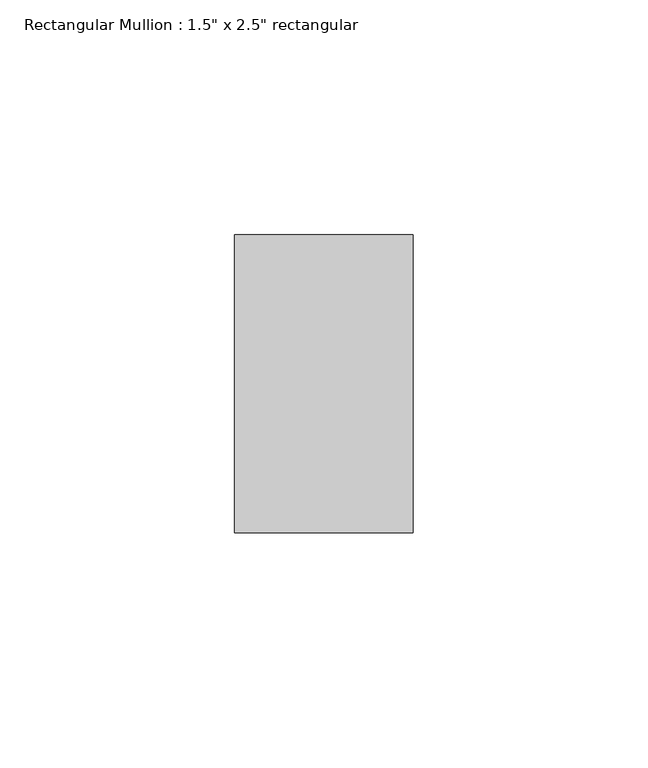
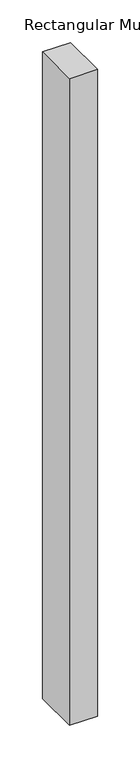
"""IFC4 building model written with IfcOpenShell, lengths in millimetres: member geometry."""

from ifc_helpers import new_model, si_unit, frame, origin, place, context, project, spatial, polyline, outline, extrude, source, transform, mapped, element, save


def member_c65a811d(model_context):
    return source(origin(), model_context, "Body", "SweptSolid", [
        extrude(outline(polyline([(0.0, 31.75), (0.0, -31.75), (-38.1, -31.75), (-38.1, 31.75), (0.0, 31.75)])), frame((0.0, 0.0, -927.1000003), z_axis=(0.0, 0.0, 1.0), x_axis=(1.0, 0.0, 0.0)), (0.0, 0.0, 1.0), 927.1000003),
    ])


if __name__ == "__main__":
    model = new_model("IFC4")
    model_context = context("Model", 3, world=origin())
    ifc_project = project(units=[si_unit("LENGTHUNIT", "METRE", prefix="MILLI")], contexts=[model_context])
    site = spatial("IfcSite", under=ifc_project)
    building = spatial("IfcBuilding", under=site)
    placement = place(None, origin())
    member_shape = member_c65a811d(model_context)
    element("IfcMember", 1, ObjectType="Rectangular Mullion : 1.5\" x 2.5\" rectangular", at=placement, inside=building, context=model_context, shape_type="MappedRepresentation", body=[
        mapped(member_shape, transform((0.0, 0.0, 0.0), x_axis=(1.0, 0.0, 0.0), y_axis=(0.0, 1.0, 0.0), z_axis=(0.0, 0.0, 1.0))),
    ])
    save(model, "model.ifc")

# Revit data of these elements
# Type "Rectangular Mullion : 1.5\" x 2.5\" rectangular"
#   built-in parameter 1007304 = 0.208333 (stored number, unit not read)
#   built-in parameter 1007301 = 0.0625 (stored number, unit not read)
#   built-in parameter 1007300 = 0.0625 (stored number, unit not read)
# Element 1 (IfcMember, "Rectangular Mullion : 1.5\" x 2.5\" rectangular")
#   Materials on its faces: "Aluminum"
# Materials
#   "Aluminum": class "Metal", colour RGB 247 247 247, transparency 0, Description = "Aluminum 6061", Cost = 0
